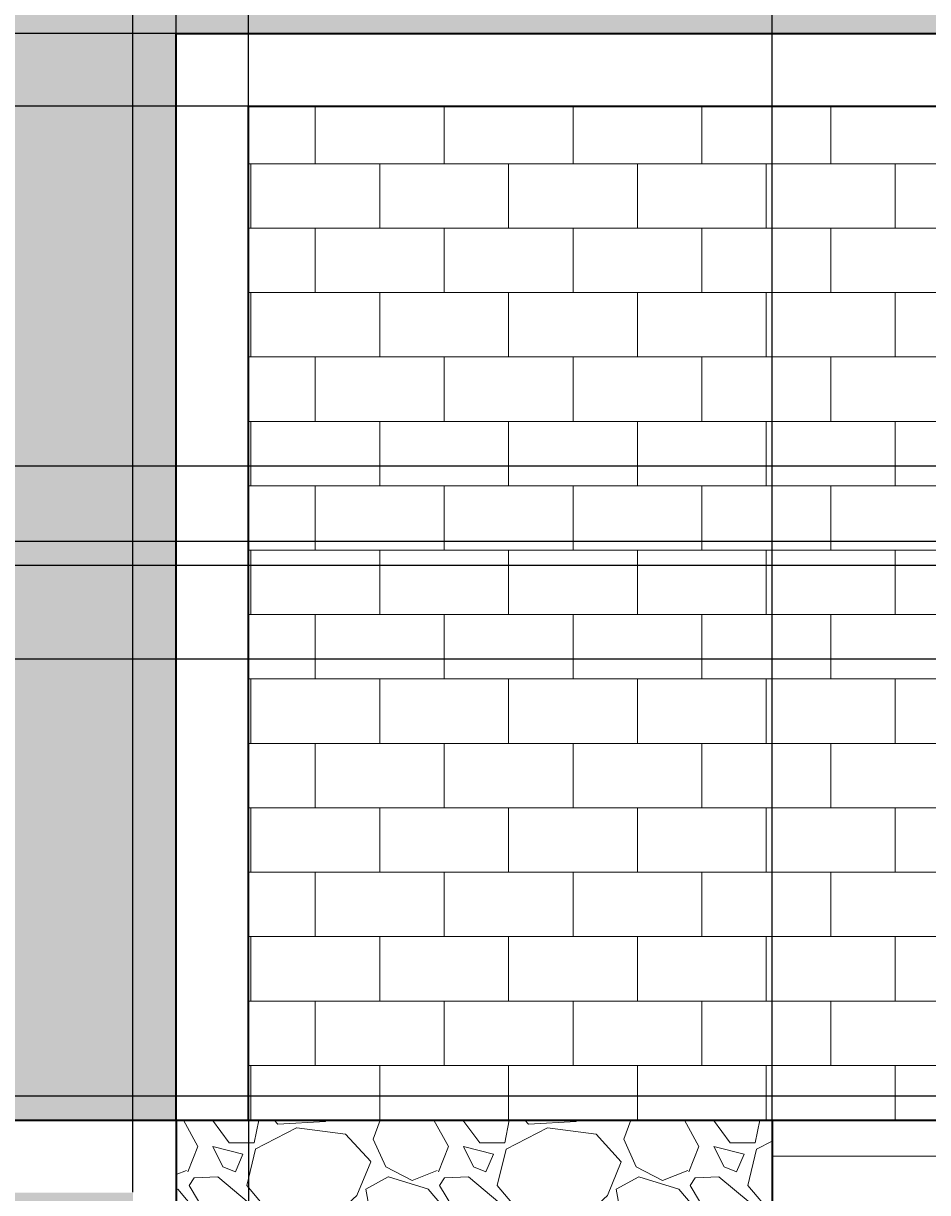
# Model space of a CAD drawing. Units: inches. Extents: x -5 to 714, y 84 to 644.
# Tile 8 of 20: x 108 to 220, y 336 to 481. Entities that reach past the tile are written whole.
import ezdxf

# ---------------------------------------------------------------- set-up
doc = ezdxf.new("R2010")
doc.units = ezdxf.units.IN
doc.header["$MEASUREMENT"] = 0
for name, color, linetype, lineweight in [('A-ANNO-DIMS', 2, 'Continuous', 18), ('A-ELEV', 7, 'Continuous', 35), ('A-ELEV-PATT', 8, 'Continuous', 13)]:
    doc.layers.add(name, color=color, linetype=linetype, lineweight=lineweight)
doc.styles.get("Standard").update_dxf_attribs({"font": 'arial.ttf'})
doc.dimstyles.get("Standard").update_dxf_attribs({"dimtxt": 0.9375, "dimasz": 0.18, "dimexe": 0.18, "dimexo": 0.0625, "dimgap": 0.09, "dimtad": 0, "dimtih": 1, "dimtoh": 1, "dimdec": 4, "dimzin": 0, "dimdsep": 46, "dimlunit": 4, "dimtxsty": 'Standard', "dimcen": 0.09, "dimadec": 0, "dimazin": 0, "dimtfac": 1, "dimtdec": 4, "dimtofl": 0, "dimtmove": 0, "dimatfit": 3, "dimfxl": 1, "dimtolj": 1, "dimtzin": 0, "dimarcsym": 0})

# ---------------------------------------------------------------- blocks, each defined once
blk = doc.blocks.new('*D16')
at = {"layer": 'A-ANNO-DIMS', "color": 0, "lineweight": -2, "transparency": 16777216}
for p, q in [((364.22, 540.29), (-2.74, 540.29)), ((-2.56, 540.11), (-2.56, 510.8)), ((-2.56, 480.35), (-2.56, 509.66)), ((364.22, 480.17), (-2.74, 480.17))]:
    blk.add_line(p, q, dxfattribs=at)
at = {"layer": 'A-ANNO-DIMS', "color": 0, "transparency": 16777216}
for points in [[(-2.59, 540.11), (-2.53, 540.11), (-2.56, 540.29)], [(-2.59, 480.35), (-2.53, 480.35), (-2.56, 480.17)]]:
    blk.add_solid(points, dxfattribs=at)
at = {"layer": 'Defpoints', "color": 0, "transparency": 16777216}
for p in [(-2.56, 540.29), (364.28, 540.29), (364.28, 480.17)]:
    blk.add_point(p, dxfattribs=at)
at = {"layer": 'A-ANNO-DIMS', "color": 0, "transparency": 16777216, "insert": (-2.56, 510.23), "char_height": 0.938, "attachment_point": 5}
blk.add_mtext('\\A1;60.11', dxfattribs=at)
blk = doc.blocks.new('*D23')
at = {"layer": 'A-ANNO-DIMS', "color": 0, "lineweight": -2, "transparency": 16777216}
for p, q in [((229.3, 525.19), (-2.74, 525.19)), ((-2.56, 525.01), (-2.56, 503.25)), ((-2.56, 480.35), (-2.56, 502.11)), ((229.3, 480.17), (-2.74, 480.17))]:
    blk.add_line(p, q, dxfattribs=at)
at = {"layer": 'A-ANNO-DIMS', "color": 0, "transparency": 16777216}
for points in [[(-2.59, 525.01), (-2.53, 525.01), (-2.56, 525.19)], [(-2.59, 480.35), (-2.53, 480.35), (-2.56, 480.17)]]:
    blk.add_solid(points, dxfattribs=at)
at = {"layer": 'Defpoints', "color": 0, "transparency": 16777216}
for p in [(-2.56, 525.19), (229.36, 525.19), (229.36, 480.17)]:
    blk.add_point(p, dxfattribs=at)
at = {"layer": 'A-ANNO-DIMS', "color": 0, "transparency": 16777216, "insert": (-2.56, 502.68), "char_height": 0.938, "attachment_point": 5}
blk.add_mtext('\\A1;45.02', dxfattribs=at)
blk = doc.blocks.new('*D24')
at = {"layer": 'A-ANNO-DIMS', "color": 0, "lineweight": -2, "transparency": 16777216}
for p, q in [((126.73, 480.23), (126.73, 643.61)), ((126.91, 643.43), (295.25, 643.43)), ((466.92, 643.43), (298.58, 643.43)), ((467.1, 480.23), (467.1, 643.61))]:
    blk.add_line(p, q, dxfattribs=at)
at = {"layer": 'A-ANNO-DIMS', "color": 0, "transparency": 16777216}
for points in [[(126.91, 643.46), (126.91, 643.4), (126.73, 643.43)], [(466.92, 643.46), (466.92, 643.4), (467.1, 643.43)]]:
    blk.add_solid(points, dxfattribs=at)
at = {"layer": 'Defpoints', "color": 0, "transparency": 16777216}
for p in [(467.1, 643.43), (126.73, 480.17), (467.1, 480.17)]:
    blk.add_point(p, dxfattribs=at)
at = {"layer": 'A-ANNO-DIMS', "color": 0, "transparency": 16777216, "insert": (296.91, 643.43), "char_height": 0.938, "attachment_point": 5}
blk.add_mtext('\\A1;340.4', dxfattribs=at)
blk = doc.blocks.new('*D25')
at = {"layer": 'A-ANNO-DIMS', "color": 0, "lineweight": -2, "transparency": 16777216}
for p, q in [((126.67, 480.17), (-2.74, 480.17)), ((-2.56, 479.99), (-2.56, 413.25)), ((-2.56, 345.37), (-2.56, 412.11)), ((126.67, 345.19), (-2.74, 345.19))]:
    blk.add_line(p, q, dxfattribs=at)
at = {"layer": 'A-ANNO-DIMS', "color": 0, "transparency": 16777216}
for points in [[(-2.59, 479.99), (-2.53, 479.99), (-2.56, 480.17)], [(-2.59, 345.37), (-2.53, 345.37), (-2.56, 345.19)]]:
    blk.add_solid(points, dxfattribs=at)
at = {"layer": 'Defpoints', "color": 0, "transparency": 16777216}
for p in [(-2.56, 480.17), (126.73, 480.17), (126.73, 345.19)]:
    blk.add_point(p, dxfattribs=at)
at = {"layer": 'A-ANNO-DIMS', "color": 0, "transparency": 16777216, "insert": (-2.56, 412.68), "char_height": 0.938, "attachment_point": 5}
blk.add_mtext('\\A1;134.98', dxfattribs=at)
blk = doc.blocks.new('*D26')
at = {"layer": 'A-ANNO-DIMS', "color": 0, "lineweight": -2, "transparency": 16777216}
for p, q in [((135.67, 471.17), (-2.74, 471.17)), ((-2.56, 470.99), (-2.56, 408.75)), ((-2.56, 345.37), (-2.56, 407.61)), ((135.67, 345.19), (-2.74, 345.19))]:
    blk.add_line(p, q, dxfattribs=at)
at = {"layer": 'A-ANNO-DIMS', "color": 0, "transparency": 16777216}
for points in [[(-2.59, 470.99), (-2.53, 470.99), (-2.56, 471.17)], [(-2.59, 345.37), (-2.53, 345.37), (-2.56, 345.19)]]:
    blk.add_solid(points, dxfattribs=at)
at = {"layer": 'Defpoints', "color": 0, "transparency": 16777216}
for p in [(-2.56, 471.17), (135.73, 471.17), (135.73, 345.19)]:
    blk.add_point(p, dxfattribs=at)
at = {"layer": 'A-ANNO-DIMS', "color": 0, "transparency": 16777216, "insert": (-2.56, 408.18), "char_height": 0.938, "attachment_point": 5}
blk.add_mtext('\\A1;125.98', dxfattribs=at)
blk = doc.blocks.new('*D27')
at = {"layer": 'A-ANNO-DIMS', "color": 0, "lineweight": -2, "transparency": 16777216}
for p, q in [((429.45, 402.48), (-2.74, 402.48)), ((-2.56, 402.3), (-2.56, 374.41)), ((-2.56, 345.37), (-2.56, 373.27)), ((429.45, 345.19), (-2.74, 345.19))]:
    blk.add_line(p, q, dxfattribs=at)
at = {"layer": 'A-ANNO-DIMS', "color": 0, "transparency": 16777216}
for points in [[(-2.59, 402.3), (-2.53, 402.3), (-2.56, 402.48)], [(-2.59, 345.37), (-2.53, 345.37), (-2.56, 345.19)]]:
    blk.add_solid(points, dxfattribs=at)
at = {"layer": 'Defpoints', "color": 0, "transparency": 16777216}
for p in [(-2.56, 402.48), (429.51, 402.48), (429.51, 345.19)]:
    blk.add_point(p, dxfattribs=at)
at = {"layer": 'A-ANNO-DIMS', "color": 0, "transparency": 16777216, "insert": (-2.56, 373.84), "char_height": 0.938, "attachment_point": 5}
blk.add_mtext('\\A1;57.29', dxfattribs=at)
blk = doc.blocks.new('*D28')
at = {"layer": 'A-ANNO-DIMS', "color": 0, "lineweight": -2, "transparency": 16777216}
for p, q in [((126.73, 480.11), (126.73, 84.31)), ((135.73, 471.11), (135.73, 84.31)), ((126.91, 84.49), (130.83, 84.49)), ((135.55, 84.49), (131.63, 84.49))]:
    blk.add_line(p, q, dxfattribs=at)
at = {"layer": 'A-ANNO-DIMS', "color": 0, "transparency": 16777216}
for points in [[(126.91, 84.52), (126.91, 84.46), (126.73, 84.49)], [(135.55, 84.52), (135.55, 84.46), (135.73, 84.49)]]:
    blk.add_solid(points, dxfattribs=at)
at = {"layer": 'Defpoints', "color": 0, "transparency": 16777216}
for p in [(126.73, 480.17), (135.73, 471.17), (135.73, 84.49)]:
    blk.add_point(p, dxfattribs=at)
at = {"layer": 'A-ANNO-DIMS', "color": 0, "transparency": 16777216, "insert": (131.23, 84.49), "char_height": 0.938, "attachment_point": 5}
blk.add_mtext('\\A1;9', dxfattribs=at)
blk = doc.blocks.new('*D29')
at = {"layer": 'A-ANNO-DIMS', "color": 0, "lineweight": -2, "transparency": 16777216}
for p, q in [((135.73, 471.11), (135.73, 84.31)), ((429.51, 471.11), (429.51, 84.31)), ((135.91, 84.49), (280.94, 84.49)), ((429.33, 84.49), (284.3, 84.49))]:
    blk.add_line(p, q, dxfattribs=at)
at = {"layer": 'A-ANNO-DIMS', "color": 0, "transparency": 16777216}
for points in [[(135.91, 84.52), (135.91, 84.46), (135.73, 84.49)], [(429.33, 84.52), (429.33, 84.46), (429.51, 84.49)]]:
    blk.add_solid(points, dxfattribs=at)
at = {"layer": 'Defpoints', "color": 0, "transparency": 16777216}
for p in [(135.73, 471.17), (429.51, 471.17), (429.51, 84.49)]:
    blk.add_point(p, dxfattribs=at)
at = {"layer": 'A-ANNO-DIMS', "color": 0, "transparency": 16777216, "insert": (282.62, 84.49), "char_height": 0.938, "attachment_point": 5}
blk.add_mtext('\\A1;293.8', dxfattribs=at)
blk = doc.blocks.new('*D31')
at = {"layer": 'A-ANNO-DIMS', "color": 0, "lineweight": -2, "transparency": 16777216}
for p, q in [((135.73, 345.26), (135.73, 643.61)), ((135.91, 643.43), (184.51, 643.43)), ((237.09, 643.43), (188.49, 643.43)), ((237.27, 345.26), (237.27, 643.61))]:
    blk.add_line(p, q, dxfattribs=at)
at = {"layer": 'A-ANNO-DIMS', "color": 0, "transparency": 16777216}
for points in [[(135.91, 643.46), (135.91, 643.4), (135.73, 643.43)], [(237.09, 643.46), (237.09, 643.4), (237.27, 643.43)]]:
    blk.add_solid(points, dxfattribs=at)
at = {"layer": 'Defpoints', "color": 0, "transparency": 16777216}
for p in [(237.27, 643.43), (135.73, 345.19), (237.27, 345.19)]:
    blk.add_point(p, dxfattribs=at)
at = {"layer": 'A-ANNO-DIMS', "color": 0, "transparency": 16777216, "insert": (186.5, 643.43), "char_height": 0.938, "attachment_point": 5}
blk.add_mtext('\\A1;101.54', dxfattribs=at)
blk = doc.blocks.new('*D34')
at = {"layer": 'A-ANNO-DIMS', "color": 0, "lineweight": -2, "transparency": 16777216}
for p, q in [((286.82, 414.09), (-2.74, 414.09)), ((-2.56, 413.91), (-2.56, 381.71)), ((-2.56, 348.37), (-2.56, 380.57)), ((286.82, 348.19), (-2.74, 348.19))]:
    blk.add_line(p, q, dxfattribs=at)
at = {"layer": 'A-ANNO-DIMS', "color": 0, "transparency": 16777216}
for points in [[(-2.59, 413.91), (-2.53, 413.91), (-2.56, 414.09)], [(-2.59, 348.37), (-2.53, 348.37), (-2.56, 348.19)]]:
    blk.add_solid(points, dxfattribs=at)
at = {"layer": 'Defpoints', "color": 0, "transparency": 16777216}
for p in [(-2.56, 414.09), (286.88, 414.09), (286.88, 348.19)]:
    blk.add_point(p, dxfattribs=at)
at = {"layer": 'A-ANNO-DIMS', "color": 0, "transparency": 16777216, "insert": (-2.56, 381.14), "char_height": 0.938, "attachment_point": 5}
blk.add_mtext('\\A1;65.9', dxfattribs=at)
blk = doc.blocks.new('*D35')
at = {"layer": 'A-ANNO-DIMS', "color": 0, "lineweight": -2, "transparency": 16777216}
for p, q in [((289.82, 417.09), (-2.74, 417.09)), ((-2.56, 416.91), (-2.56, 381.71)), ((-2.56, 345.37), (-2.56, 380.57)), ((289.82, 345.19), (-2.74, 345.19))]:
    blk.add_line(p, q, dxfattribs=at)
at = {"layer": 'A-ANNO-DIMS', "color": 0, "transparency": 16777216}
for points in [[(-2.59, 416.91), (-2.53, 416.91), (-2.56, 417.09)], [(-2.59, 345.37), (-2.53, 345.37), (-2.56, 345.19)]]:
    blk.add_solid(points, dxfattribs=at)
at = {"layer": 'Defpoints', "color": 0, "transparency": 16777216}
for p in [(-2.56, 417.09), (289.88, 417.09), (289.88, 345.19)]:
    blk.add_point(p, dxfattribs=at)
at = {"layer": 'A-ANNO-DIMS', "color": 0, "transparency": 16777216, "insert": (-2.56, 381.14), "char_height": 0.938, "attachment_point": 5}
blk.add_mtext('\\A1;71.9', dxfattribs=at)
blk = doc.blocks.new('*D37')
at = {"layer": 'A-ANNO-DIMS', "color": 0, "lineweight": -2, "transparency": 16777216}
for p, q in [((302.44, 426.45), (-2.74, 426.45)), ((-2.56, 426.27), (-2.56, 422.34)), ((-2.56, 417.27), (-2.56, 421.2)), ((302.44, 417.09), (-2.74, 417.09))]:
    blk.add_line(p, q, dxfattribs=at)
at = {"layer": 'A-ANNO-DIMS', "color": 0, "transparency": 16777216}
for points in [[(-2.59, 426.27), (-2.53, 426.27), (-2.56, 426.45)], [(-2.59, 417.27), (-2.53, 417.27), (-2.56, 417.09)]]:
    blk.add_solid(points, dxfattribs=at)
at = {"layer": 'Defpoints', "color": 0, "transparency": 16777216}
for p in [(-2.56, 426.45), (302.5, 426.45), (302.5, 417.09)]:
    blk.add_point(p, dxfattribs=at)
at = {"layer": 'A-ANNO-DIMS', "color": 0, "transparency": 16777216, "insert": (-2.56, 421.77), "char_height": 0.938, "attachment_point": 5}
blk.add_mtext('\\A1;9.358', dxfattribs=at)
blk = doc.blocks.new('*D47')
at = {"layer": 'A-ANNO-DIMS', "color": 0, "lineweight": -2, "transparency": 16777216}
for p, q in [((75.5, 336.27), (75.5, 643.61)), ((75.68, 643.43), (96.74, 643.43)), ((121.18, 643.43), (100.13, 643.43)), ((121.36, 336.27), (121.36, 643.61))]:
    blk.add_line(p, q, dxfattribs=at)
at = {"layer": 'A-ANNO-DIMS', "color": 0, "transparency": 16777216}
for points in [[(75.68, 643.46), (75.68, 643.4), (75.5, 643.43)], [(121.18, 643.46), (121.18, 643.4), (121.36, 643.43)]]:
    blk.add_solid(points, dxfattribs=at)
at = {"layer": 'Defpoints', "color": 0, "transparency": 16777216}
for p in [(121.36, 643.43), (75.5, 336.21), (121.36, 336.21)]:
    blk.add_point(p, dxfattribs=at)
at = {"layer": 'A-ANNO-DIMS', "color": 0, "transparency": 16777216, "insert": (98.43, 643.43), "char_height": 0.938, "attachment_point": 5}
blk.add_mtext('\\A1;45.85', dxfattribs=at)
blk = doc.blocks.new('*D48')
at = {"layer": 'A-ANNO-DIMS', "color": 0, "lineweight": -2, "transparency": 16777216}
for p, q in [((121.36, 336.27), (121.36, 643.61)), ((121.54, 643.43), (122.46, 643.43)), ((126.55, 643.43), (125.63, 643.43)), ((126.73, 345.26), (126.73, 643.61))]:
    blk.add_line(p, q, dxfattribs=at)
at = {"layer": 'A-ANNO-DIMS', "color": 0, "transparency": 16777216}
for points in [[(121.54, 643.46), (121.54, 643.4), (121.36, 643.43)], [(126.55, 643.46), (126.55, 643.4), (126.73, 643.43)]]:
    blk.add_solid(points, dxfattribs=at)
at = {"layer": 'Defpoints', "color": 0, "transparency": 16777216}
for p in [(126.73, 643.43), (126.73, 345.19), (121.36, 336.21)]:
    blk.add_point(p, dxfattribs=at)
at = {"layer": 'A-ANNO-DIMS', "color": 0, "transparency": 16777216, "insert": (124.04, 643.43), "char_height": 0.938, "attachment_point": 5}
blk.add_mtext('\\A1;5.371', dxfattribs=at)
blk = doc.blocks.new('*D49')
at = {"layer": 'A-ANNO-DIMS', "color": 0, "lineweight": -2, "transparency": 16777216}
for p, q in [((126.73, 302), (126.73, 643.61)), ((126.91, 643.43), (162.98, 643.43)), ((200.56, 643.43), (164.49, 643.43)), ((200.74, 302), (200.74, 643.61))]:
    blk.add_line(p, q, dxfattribs=at)
at = {"layer": 'A-ANNO-DIMS', "color": 0, "transparency": 16777216}
for points in [[(126.91, 643.46), (126.91, 643.4), (126.73, 643.43)], [(200.56, 643.46), (200.56, 643.4), (200.74, 643.43)]]:
    blk.add_solid(points, dxfattribs=at)
at = {"layer": 'Defpoints', "color": 0, "transparency": 16777216}
for p in [(200.74, 643.43), (126.73, 301.94), (200.74, 301.94)]:
    blk.add_point(p, dxfattribs=at)
at = {"layer": 'A-ANNO-DIMS', "color": 0, "transparency": 16777216, "insert": (163.73, 643.43), "char_height": 0.938, "attachment_point": 5}
blk.add_mtext('\\A1;74', dxfattribs=at)
blk = doc.blocks.new('*D50')
at = {"layer": 'A-ANNO-DIMS', "color": 0, "lineweight": -2, "transparency": 16777216}
for p, q in [((200.67, 345.19), (-2.74, 345.19)), ((-2.56, 345.01), (-2.56, 324.13)), ((-2.56, 302.12), (-2.56, 323)), ((200.67, 301.94), (-2.74, 301.94))]:
    blk.add_line(p, q, dxfattribs=at)
at = {"layer": 'A-ANNO-DIMS', "color": 0, "transparency": 16777216}
for points in [[(-2.59, 345.01), (-2.53, 345.01), (-2.56, 345.19)], [(-2.59, 302.12), (-2.53, 302.12), (-2.56, 301.94)]]:
    blk.add_solid(points, dxfattribs=at)
at = {"layer": 'Defpoints', "color": 0, "transparency": 16777216}
for p in [(-2.56, 345.19), (200.74, 345.19), (200.74, 301.94)]:
    blk.add_point(p, dxfattribs=at)
at = {"layer": 'A-ANNO-DIMS', "color": 0, "transparency": 16777216, "insert": (-2.56, 323.57), "char_height": 0.938, "attachment_point": 5}
blk.add_mtext('\\A1;43.255', dxfattribs=at)
blk = doc.blocks.new('*D51')
at = {"layer": 'A-ANNO-DIMS', "color": 0, "lineweight": -2, "transparency": 16777216}
for p, q in [((200.74, 201.26), (200.74, 643.61)), ((200.92, 643.43), (223.39, 643.43)), ((249.24, 643.43), (226.77, 643.43)), ((249.42, 201.26), (249.42, 643.61))]:
    blk.add_line(p, q, dxfattribs=at)
at = {"layer": 'A-ANNO-DIMS', "color": 0, "transparency": 16777216}
for points in [[(200.92, 643.46), (200.92, 643.4), (200.74, 643.43)], [(249.24, 643.46), (249.24, 643.4), (249.42, 643.43)]]:
    blk.add_solid(points, dxfattribs=at)
at = {"layer": 'Defpoints', "color": 0, "transparency": 16777216}
for p in [(249.42, 643.43), (200.74, 201.19), (249.42, 201.19)]:
    blk.add_point(p, dxfattribs=at)
at = {"layer": 'A-ANNO-DIMS', "color": 0, "transparency": 16777216, "insert": (225.08, 643.43), "char_height": 0.938, "attachment_point": 5}
blk.add_mtext('\\A1;48.68', dxfattribs=at)

msp = doc.modelspace()

# ---------------------------------------------------------------- hatches: boundary and pattern name
at = {"layer": 'A-ELEV-PATT', "transparency": 33554687}
h = msp.add_hatch(color=256, dxfattribs=at)
h.dxf.hatch_style = 1
h.paths.add_polyline_path([(188.3677, 525.1928), (67.9893, 525.1928), (67.9893, 489.1928), (67.9893, 345.1928), (126.7303, 345.1928), (126.7303, 480.1709), (229.3575, 480.1709), (229.3575, 525.1928), (212.6043, 525.1928), (212.6043, 482.7164), (211.0019, 482.7164), (211.0019, 525.1928), (207.6919, 525.1928), (199.9852, 525.1928), (199.9852, 482.7164), (198.3828, 482.7164), (198.3828, 525.1928), (189.9701, 525.1928), (189.9701, 482.7164), (188.3677, 482.7164)])
h.paths.add_polyline_path([(121.3589, 336.2066), (75.5048, 336.2066), (75.5048, 319.345), (121.3589, 319.345)])
h.paths.add_polyline_path([(121.3589, 319.345), (75.5048, 319.345), (75.5048, 302.3045), (121.3589, 302.3045)])
h.paths.add_polyline_path([(121.3589, 302.3045), (75.5048, 302.3045), (75.5048, 282.8561), (121.3589, 282.8561)])
h.paths.add_polyline_path([(121.3589, 282.8561), (75.5048, 282.8561), (75.5048, 261.5556), (121.3589, 261.5556)])
h.paths.add_polyline_path([(121.3589, 261.5556), (75.5048, 261.5556), (75.5048, 243.7009), (121.3589, 243.7009)])
h.paths.add_polyline_path([(121.3589, 243.7009), (75.5048, 243.7009), (75.5048, 223.5117), (121.3589, 223.5117)])
h.paths.add_polyline_path([(121.3589, 223.5117), (75.5048, 223.5117), (75.5048, 212.5836), (121.3589, 212.5836)])
h.paths.add_polyline_path([(121.3589, 212.5836), (75.5048, 212.5836), (75.5048, 201.1928), (121.3589, 201.1928)])
h.paths.add_polyline_path([(179.9335, 201.1928), (30.1395, 201.1928), (30.1395, 198.7054), (179.9335, 198.7054)])
h.paths.add_polyline_path([(187.6349, 201.1928), (179.9335, 201.1928), (179.9335, 198.7054), (179.9335, 141.1928), (269.2446, 141.1928), (269.2446, 201.1928), (263.4349, 201.1928), (263.4349, 152.1176), (187.6349, 152.1176)])
h.paths.add_polyline_path([(269.2446, 277.0513), (269.2446, 287.501), (269.2446, 306.6286), (578.0915, 306.6286), (578.0915, 201.1928), (593.428, 201.1928), (593.428, 315.0968), (584.4202, 315.0968), (259.0665, 315.0968), (259.0665, 201.1928), (263.4349, 201.1928), (269.2446, 201.1928)])
h = msp.add_hatch(dxfattribs=at)
h.set_pattern_fill('ANSI31', color=256, scale=58, angle=135)
h.paths.add_polyline_path([(249.4181, 345.1928), (237.2654, 345.1928), (200.7361, 345.1928), (200.7361, 201.1928), (249.4181, 201.1928)])
h.paths.add_polyline_path([(261.4349, 199.1928), (189.6349, 199.1928), (189.6349, 154.1176), (261.4349, 154.1176)])
h.paths.add_polyline_path([(415.8092, 525.1928), (366.2809, 525.1928), (366.2809, 480.1709), (415.8092, 480.1709)])
h = msp.add_hatch(dxfattribs=at)
h.set_pattern_fill('AR-B816', color=256)
h.paths.add_polyline_path([(429.5094, 471.1709), (412.7784, 471.1709), (229.3575, 471.1709), (135.7303, 471.1709), (135.7303, 345.1928), (237.2654, 345.1928), (237.2654, 417.0908), (224.6446, 417.0908), (224.6446, 426.4485), (302.5023, 426.4485), (302.5023, 417.0908), (289.8815, 417.0908), (289.8815, 345.1928), (429.5094, 345.1928)])
h = msp.add_hatch(dxfattribs=at)
h.set_pattern_fill('GRAVEL', color=256, scale=22, angle=135)
h.paths.add_polyline_path([(200.7361, 345.1928), (126.7303, 345.1928), (126.7303, 301.9374), (200.7361, 301.9374)])

# ---------------------------------------------------------------- linework, layer by layer
at = {"layer": 'A-ELEV'}
for p, q in [((126.7303, 345.1928), (126.7303, 480.1709)), ((126.7303, 480.1709), (229.3575, 480.1709)), ((135.7303, 345.1928), (135.7303, 471.1709)), ((135.7303, 471.1709), (229.3575, 471.1709)), ((67.9893, 345.1928), (587.5794, 345.1928)), ((126.7303, 345.1928), (126.7303, 201.1928)), ((200.7361, 345.1928), (200.7361, 201.1928))]:
    msp.add_line(p, q, dxfattribs=at)

# ---------------------------------------------------------------- dimensions: what is measured, and where the dimension line sits
at = {"layer": 'A-ANNO-DIMS'}
for base, p1, p2, override, picture, middle in [((121.3589, 643.4276), (75.5048, 336.2066), (121.3589, 336.2066), {"dimdec": 2, "dimlfac": 1, "dimrnd": 0, "dimzin": 0, "dimdsep": 46, "dimlunit": 2}, '*D47', (98.4319, 643.4276)), ((126.7303, 643.4276), (121.3589, 336.2066), (126.7303, 345.1928), {"dimdec": 3, "dimlfac": 1, "dimrnd": 0, "dimzin": 0, "dimdsep": 46, "dimlunit": 2}, '*D48', (124.0446, 643.4276)), ((467.0994, 643.4276), (126.7303, 480.1709), (467.0994, 480.1709), {"dimdec": 1, "dimlfac": 1, "dimrnd": 0, "dimzin": 0, "dimdsep": 46, "dimlunit": 2}, '*D24', (296.9148, 643.4276)), ((200.7361, 643.4276), (126.7303, 301.9374), (200.7361, 301.9374), {"dimdec": 0, "dimlfac": 1, "dimrnd": 0, "dimzin": 0, "dimdsep": 46, "dimlunit": 2}, '*D49', (163.7332, 643.4276)), ((237.2654, 643.4276), (135.7303, 345.1928), (237.2654, 345.1928), {"dimdec": 2, "dimlfac": 1, "dimrnd": 0, "dimzin": 0, "dimdsep": 46, "dimlunit": 2}, '*D31', (186.4978, 643.4276)), ((249.4181, 643.4276), (200.7361, 201.1928), (249.4181, 201.1928), {"dimdec": 2, "dimlfac": 1, "dimrnd": 0, "dimzin": 0, "dimdsep": 46, "dimlunit": 2}, '*D51', (225.0771, 643.4276)), ((135.7303, 84.4928), (126.7303, 480.1709), (135.7303, 471.1709), {"dimdec": 0, "dimlfac": 1, "dimrnd": 0, "dimzin": 0, "dimdsep": 46, "dimlunit": 2}, '*D28', (131.2303, 84.4928)), ((429.5094, 84.4928), (135.7303, 471.1709), (429.5094, 471.1709), {"dimdec": 1, "dimlfac": 1, "dimrnd": 0, "dimzin": 0, "dimdsep": 46, "dimlunit": 2}, '*D29', (282.6198, 84.4928))]:
    dim = msp.add_linear_dim(base=base, p1=p1, p2=p2, dimstyle='Standard', override=override, dxfattribs=at)
    dim.commit()
    dim.dimension.update_dxf_attribs({"geometry": picture, "text_midpoint": middle})
for base, p1, p2, override, picture, middle in [((-2.5605, 540.2857), (364.2809, 480.1709), (364.2809, 540.2857), {"dimdec": 2, "dimlfac": 1, "dimrnd": 0, "dimzin": 0, "dimdsep": 46, "dimlunit": 2}, '*D16', (-2.5605, 510.2283)), ((-2.5605, 525.1928), (229.3575, 480.1709), (229.3575, 525.1928), {"dimdec": 2, "dimlfac": 1, "dimrnd": 0, "dimzin": 0, "dimdsep": 46, "dimlunit": 2}, '*D23', (-2.5605, 502.6819)), ((-2.5605, 480.1709), (126.7303, 345.1928), (126.7303, 480.1709), {"dimdec": 2, "dimlfac": 1, "dimrnd": 0, "dimzin": 0, "dimdsep": 46, "dimlunit": 2}, '*D25', (-2.5605, 412.6819)), ((-2.5605, 471.1709), (135.7303, 345.1928), (135.7303, 471.1709), {"dimdec": 2, "dimlfac": 1, "dimrnd": 0, "dimzin": 0, "dimdsep": 46, "dimlunit": 2}, '*D26', (-2.5605, 408.1819)), ((-2.5605, 426.4485), (302.5023, 417.0908), (302.5023, 426.4485), {"dimdec": 3, "dimlfac": 1, "dimrnd": 0, "dimzin": 0, "dimdsep": 46, "dimlunit": 2}, '*D37', (-2.5605, 421.7696)), ((-2.5605, 417.0908), (289.8815, 345.1928), (289.8815, 417.0908), {"dimdec": 1, "dimlfac": 1, "dimrnd": 0, "dimzin": 0, "dimdsep": 46, "dimlunit": 2}, '*D35', (-2.5605, 381.1418)), ((-2.5605, 414.0908), (286.8815, 348.1928), (286.8815, 414.0908), {"dimdec": 1, "dimlfac": 1, "dimrnd": 0, "dimzin": 0, "dimdsep": 46, "dimlunit": 2}, '*D34', (-2.5605, 381.1418)), ((-2.5605, 402.4806), (429.5094, 345.1928), (429.5094, 402.4806), {"dimdec": 2, "dimlfac": 1, "dimrnd": 0, "dimzin": 0, "dimdsep": 46, "dimlunit": 2}, '*D27', (-2.5605, 373.8367)), ((-2.5605, 345.1928), (200.7361, 301.9374), (200.7361, 345.1928), {"dimdec": 3, "dimlfac": 1, "dimrnd": 0, "dimzin": 0, "dimdsep": 46, "dimlunit": 2}, '*D50', (-2.5605, 323.5651))]:
    dim = msp.add_linear_dim(base=base, p1=p1, p2=p2, angle=90, dimstyle='Standard', override=override, dxfattribs=at)
    dim.commit()
    dim.dimension.update_dxf_attribs({"geometry": picture, "text_midpoint": middle})

doc.saveas('drawing.dxf')
